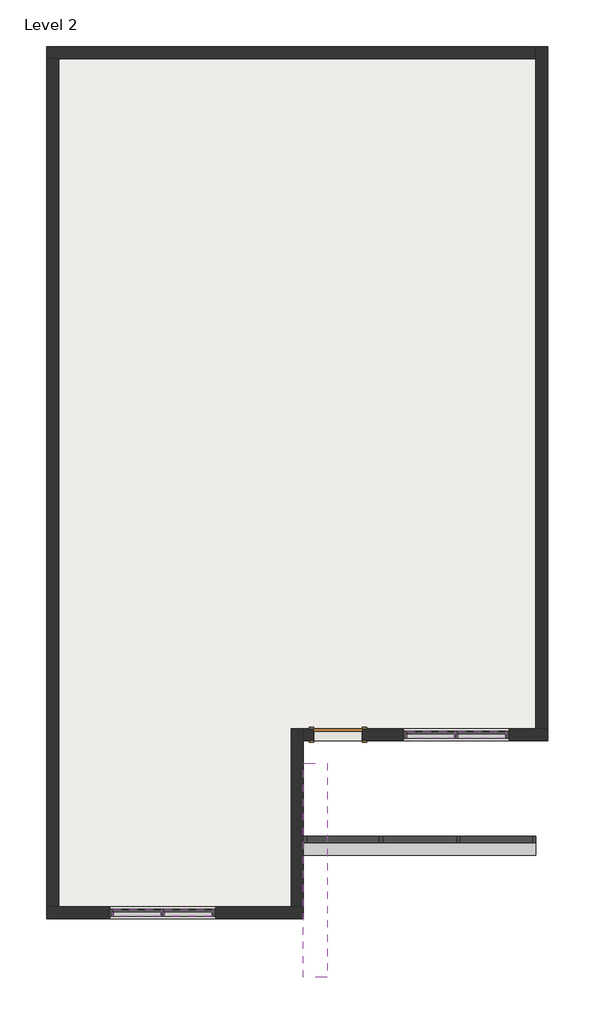
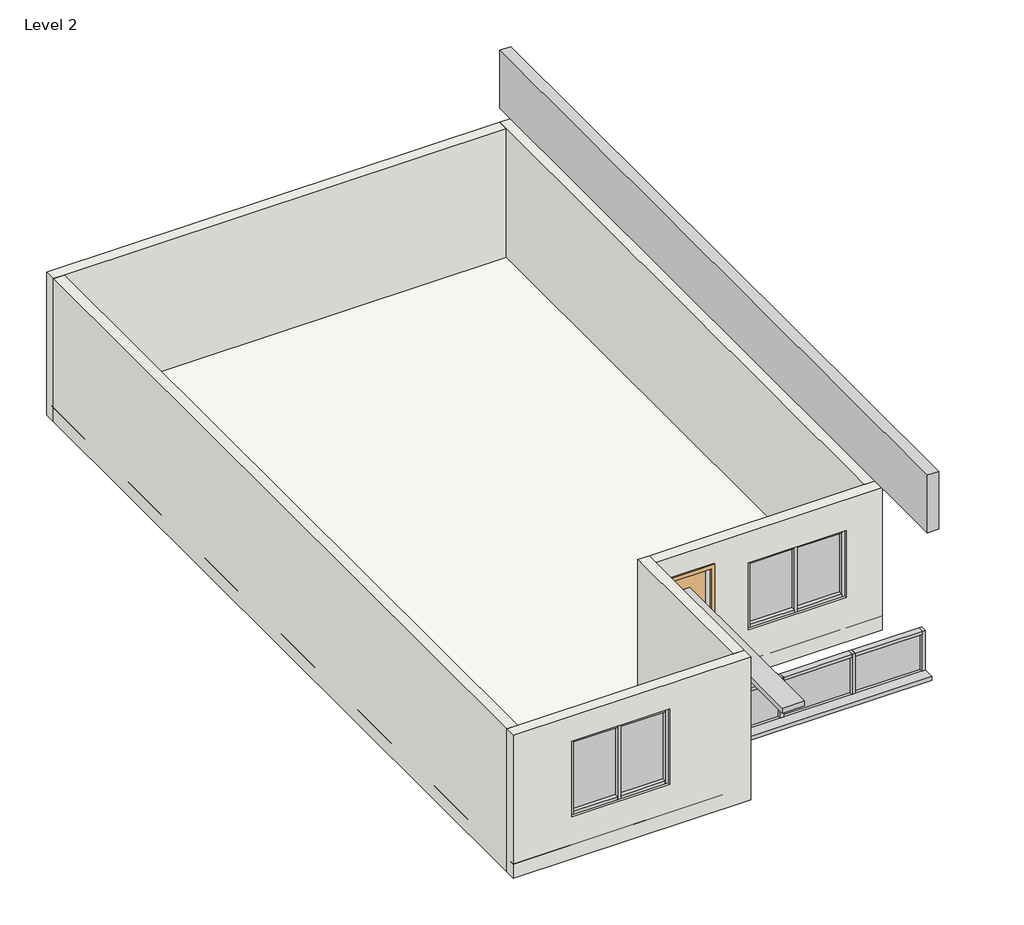
# One storey: 24 members, 7 plates, 6 walls, 2 proxies, 1 door, 1 roof.
"""IFC4 building model written with IfcOpenShell, lengths in millimetres."""

from ifc_helpers import new_model, si_unit, frame, origin, place, context, project, spatial, polyline, outline, extrude, faceted_brep, transform, mapped, element, save
from components import generic_models_2_generic_models_2_9dd516d1, generic_models_3_generic_models_3_6894cc3d, door_0ca8825f, member_f1f71bde, member_1afc5165, member_5bd926c3, member_c72ed4d9, member_c6cbf9be, member_20eb5ac3, member_846957be, member_d3800c19, member_e1cf819f, system_panel_glazed_d3edc084, system_panel_glazed_88eb0887, system_panel_glazed_baedfebd, system_panel_glazed_353e56bd

model = new_model("IFC4")

# Units and contexts
model_context = context("Model", 3, world=origin())
ifc_project = project(units=[si_unit("LENGTHUNIT", "METRE", prefix="MILLI")], contexts=[model_context])

# Site, building, storey
site = spatial("IfcSite", under=ifc_project)
building = spatial("IfcBuilding", under=site)
storey = spatial("IfcBuildingStorey", under=building, Name="Level 2", Elevation=3048.0)

# Proxies
placement = place(None, origin())
generic_models_2_generic_models_2_shape = generic_models_2_generic_models_2_9dd516d1(model_context)
element("IfcBuildingElementProxy", 1, Name="Generic Models 2 : Generic Models 2", ObjectType="Generic Models 2 : Generic Models 2", at=placement, inside=storey, context=model_context, shape_type="MappedRepresentation", body=[
    mapped(generic_models_2_generic_models_2_shape, transform((0.0, 0.0, 0.0), x_axis=(1.0, 0.0, 0.0), y_axis=(0.0, 1.0, 0.0), z_axis=(0.0, 0.0, 1.0))),
])
generic_models_3_generic_models_3_shape = generic_models_3_generic_models_3_6894cc3d(model_context)
element("IfcBuildingElementProxy", 2, Name="Generic Models 3 : Generic Models 3", ObjectType="Generic Models 3 : Generic Models 3", at=placement, inside=storey, context=model_context, shape_type="MappedRepresentation", body=[
    mapped(generic_models_3_generic_models_3_shape, transform((0.0, 0.0, 0.0), x_axis=(1.0, 0.0, 0.0), y_axis=(0.0, 1.0, 0.0), z_axis=(0.0, 0.0, 1.0))),
])

# Door
door_shape = door_0ca8825f(model_context)
element("IfcDoor", 3, ObjectType="Single-Flush : 36\" x 84\"", at=placement, inside=storey, context=model_context, shape_type="MappedRepresentation", body=[
    mapped(door_shape, transform((-14644.7161422, -7377.2867758, 3454.4), x_axis=(1.0, 0.0, 0.0), y_axis=(0.0, 1.0, 0.0), z_axis=(0.0, 0.0, 1.0))),
])

# Members
member_shape = member_f1f71bde(model_context)
element("IfcMember", 4, ObjectType="Rectangular Mullion : 2.5\" x 5\" rectangular", at=placement, inside=storey, context=model_context, shape_type="MappedRepresentation", body=[
    mapped(member_shape, transform((-17889.5661422, -10704.6867758, 3945.1177063), x_axis=(0.0, 0.0, -1.0), y_axis=(0.0, -1.0, 0.0), z_axis=(-1.0, 0.0, 0.0))),
])
element("IfcMember", 5, ObjectType="Rectangular Mullion : 2.5\" x 5\" rectangular", at=placement, inside=storey, context=model_context, shape_type="MappedRepresentation", body=[
    mapped(member_shape, transform((-18848.4161422, -10704.6867758, 3945.1177063), x_axis=(0.0, 0.0, -1.0), y_axis=(0.0, -1.0, 0.0), z_axis=(-1.0, 0.0, 0.0))),
])
element("IfcMember", 6, ObjectType="Rectangular Mullion : 2.5\" x 5\" rectangular", at=placement, inside=storey, context=model_context, shape_type="MappedRepresentation", body=[
    mapped(member_shape, transform((-12403.1661422, -7377.2867758, 3998.6028627), x_axis=(0.0, 0.0, -1.0), y_axis=(0.0, -1.0, 0.0), z_axis=(-1.0, 0.0, 0.0))),
])
element("IfcMember", 7, ObjectType="Rectangular Mullion : 2.5\" x 5\" rectangular", at=placement, inside=storey, context=model_context, shape_type="MappedRepresentation", body=[
    mapped(member_shape, transform((-13362.0161422, -7377.2867758, 3998.6028627), x_axis=(0.0, 0.0, -1.0), y_axis=(0.0, -1.0, 0.0), z_axis=(-1.0, 0.0, 0.0))),
])
element("IfcMember", 8, ObjectType="Rectangular Mullion : 2.5\" x 5\" rectangular", at=placement, inside=storey, context=model_context, shape_type="MappedRepresentation", body=[
    mapped(member_shape, transform((-17953.0661422, -10704.6867758, 5554.6402073), x_axis=(0.0, 0.0, 1.0), y_axis=(0.0, -1.0, 0.0), z_axis=(1.0, 0.0, 0.0))),
])
element("IfcMember", 9, ObjectType="Rectangular Mullion : 2.5\" x 5\" rectangular", at=placement, inside=storey, context=model_context, shape_type="MappedRepresentation", body=[
    mapped(member_shape, transform((-16994.2161422, -10704.6867758, 5554.6402073), x_axis=(0.0, 0.0, 1.0), y_axis=(0.0, -1.0, 0.0), z_axis=(1.0, 0.0, 0.0))),
])
element("IfcMember", 10, ObjectType="Rectangular Mullion : 2.5\" x 5\" rectangular", at=placement, inside=storey, context=model_context, shape_type="MappedRepresentation", body=[
    mapped(member_shape, transform((-12466.6661422, -7377.2867758, 5431.5526731), x_axis=(0.0, 0.0, 1.0), y_axis=(0.0, -1.0, 0.0), z_axis=(1.0, 0.0, 0.0))),
])
element("IfcMember", 11, ObjectType="Rectangular Mullion : 2.5\" x 5\" rectangular", at=placement, inside=storey, context=model_context, shape_type="MappedRepresentation", body=[
    mapped(member_shape, transform((-11507.8161422, -7377.2867758, 5431.5526731), x_axis=(0.0, 0.0, 1.0), y_axis=(0.0, -1.0, 0.0), z_axis=(1.0, 0.0, 0.0))),
])
member_2_shape = member_1afc5165(model_context)
element("IfcMember", 12, ObjectType="Rectangular Mullion : 2.5\" x 5\" rectangular", at=placement, inside=storey, context=model_context, shape_type="MappedRepresentation", body=[
    mapped(member_2_shape, transform((-17921.3161422, -10704.6867758, 3945.1177063), x_axis=(1.0, 0.0, 0.0), y_axis=(0.0, -1.0, 0.0), z_axis=(0.0, 0.0, -1.0))),
])
member_3_shape = member_5bd926c3(model_context)
element("IfcMember", 13, ObjectType="Rectangular Mullion : 2.5\" x 5\" rectangular", at=placement, inside=storey, context=model_context, shape_type="MappedRepresentation", body=[
    mapped(member_3_shape, transform((-18911.9161422, -10704.6867758, 5554.6402073), x_axis=(-1.0, 0.0, 0.0), y_axis=(0.0, -1.0, 0.0), z_axis=(0.0, 0.0, 1.0))),
])
element("IfcMember", 14, ObjectType="Rectangular Mullion : 2.5\" x 5\" rectangular", at=placement, inside=storey, context=model_context, shape_type="MappedRepresentation", body=[
    mapped(member_3_shape, transform((-16930.7161422, -10704.6867758, 3945.1177063), x_axis=(1.0, 0.0, 0.0), y_axis=(0.0, -1.0, 0.0), z_axis=(0.0, 0.0, -1.0))),
])
member_4_shape = member_c72ed4d9(model_context)
element("IfcMember", 15, ObjectType="Rectangular Mullion : 2.5\" x 5\" rectangular", at=placement, inside=storey, context=model_context, shape_type="MappedRepresentation", body=[
    mapped(member_4_shape, transform((-12434.9161422, -7377.2867758, 3998.6028627), x_axis=(1.0, 0.0, 0.0), y_axis=(0.0, -1.0, 0.0), z_axis=(0.0, 0.0, -1.0))),
])
member_5_shape = member_c6cbf9be(model_context)
element("IfcMember", 16, ObjectType="Rectangular Mullion : 2.5\" x 5\" rectangular", at=placement, inside=storey, context=model_context, shape_type="MappedRepresentation", body=[
    mapped(member_5_shape, transform((-13425.5161422, -7377.2867758, 5431.5526731), x_axis=(-1.0, 0.0, 0.0), y_axis=(0.0, -1.0, 0.0), z_axis=(0.0, 0.0, 1.0))),
])
element("IfcMember", 17, ObjectType="Rectangular Mullion : 2.5\" x 5\" rectangular", at=placement, inside=storey, context=model_context, shape_type="MappedRepresentation", body=[
    mapped(member_5_shape, transform((-11444.3161422, -7377.2867758, 3998.6028627), x_axis=(1.0, 0.0, 0.0), y_axis=(0.0, -1.0, 0.0), z_axis=(0.0, 0.0, -1.0))),
])
member_6_shape = member_20eb5ac3(model_context)
element("IfcMember", 18, ObjectType="Rectangular Mullion : 2.5\" x 5\" rectangular", at=placement, inside=storey, context=model_context, shape_type="MappedRepresentation", body=[
    mapped(member_6_shape, transform((-13876.3661422, -9333.0867758, 4278.7054943), x_axis=(0.0, 0.0, 1.0), y_axis=(0.0, -1.0, 0.0), z_axis=(1.0, 0.0, 0.0))),
])
element("IfcMember", 19, ObjectType="Rectangular Mullion : 2.5\" x 5\" rectangular", at=placement, inside=storey, context=model_context, shape_type="MappedRepresentation", body=[
    mapped(member_6_shape, transform((-11012.5161422, -9333.0867758, 4278.7054943), x_axis=(0.0, 0.0, 1.0), y_axis=(0.0, -1.0, 0.0), z_axis=(1.0, 0.0, 0.0))),
])
member_7_shape = member_846957be(model_context)
element("IfcMember", 20, ObjectType="Rectangular Mullion : 2.5\" x 5\" rectangular", at=placement, inside=storey, context=model_context, shape_type="MappedRepresentation", body=[
    mapped(member_7_shape, transform((-13844.6161422, -9333.0867758, 3352.8), x_axis=(1.0, 0.0, 0.0), y_axis=(0.0, -1.0, 0.0), z_axis=(0.0, 0.0, -1.0))),
])
element("IfcMember", 21, ObjectType="Rectangular Mullion : 2.5\" x 5\" rectangular", at=placement, inside=storey, context=model_context, shape_type="MappedRepresentation", body=[
    mapped(member_7_shape, transform((-12396.8161422, -9333.0867758, 3352.8), x_axis=(1.0, 0.0, 0.0), y_axis=(0.0, -1.0, 0.0), z_axis=(0.0, 0.0, -1.0))),
])
element("IfcMember", 22, ObjectType="Rectangular Mullion : 2.5\" x 5\" rectangular", at=placement, inside=storey, context=model_context, shape_type="MappedRepresentation", body=[
    mapped(member_6_shape, transform((-12365.0661422, -9333.0867758, 3352.8), x_axis=(0.0, 0.0, -1.0), y_axis=(0.0, -1.0, 0.0), z_axis=(-1.0, 0.0, 0.0))),
])
element("IfcMember", 23, ObjectType="Rectangular Mullion : 2.5\" x 5\" rectangular", at=placement, inside=storey, context=model_context, shape_type="MappedRepresentation", body=[
    mapped(member_6_shape, transform((-15228.9161422, -9333.0867758, 3352.8), x_axis=(0.0, 0.0, -1.0), y_axis=(0.0, -1.0, 0.0), z_axis=(-1.0, 0.0, 0.0))),
])
member_8_shape = member_d3800c19(model_context)
element("IfcMember", 24, ObjectType="Rectangular Mullion : 2.5\" x 5\" rectangular", at=placement, inside=storey, context=model_context, shape_type="MappedRepresentation", body=[
    mapped(member_8_shape, transform((-15292.4161422, -9333.0867758, 4278.7054943), x_axis=(-1.0, 0.0, 0.0), y_axis=(0.0, -1.0, 0.0), z_axis=(0.0, 0.0, 1.0))),
])
member_9_shape = member_e1cf819f(model_context)
element("IfcMember", 25, ObjectType="Rectangular Mullion : 2.5\" x 5\" rectangular", at=placement, inside=storey, context=model_context, shape_type="MappedRepresentation", body=[
    mapped(member_9_shape, transform((-12428.5661422, -9333.0867758, 4278.7054943), x_axis=(0.0, 0.0, 1.0), y_axis=(0.0, -1.0, 0.0), z_axis=(1.0, 0.0, 0.0))),
])
element("IfcMember", 26, ObjectType="Rectangular Mullion : 2.5\" x 5\" rectangular", at=placement, inside=storey, context=model_context, shape_type="MappedRepresentation", body=[
    mapped(member_9_shape, transform((-13812.8661422, -9333.0867758, 3352.8), x_axis=(0.0, 0.0, -1.0), y_axis=(0.0, -1.0, 0.0), z_axis=(-1.0, 0.0, 0.0))),
])
element("IfcMember", 27, ObjectType="Rectangular Mullion : 2.5\" x 5\" rectangular", at=placement, inside=storey, context=model_context, shape_type="MappedRepresentation", body=[
    mapped(member_8_shape, transform((-10949.0161422, -9333.0867758, 3352.8), x_axis=(1.0, 0.0, 0.0), y_axis=(0.0, -1.0, 0.0), z_axis=(0.0, 0.0, -1.0))),
])

# Plates
system_panel_glazed_shape = system_panel_glazed_d3edc084(model_context)
element("IfcPlate", 28, ObjectType="System Panel : Glazed", at=placement, inside=storey, context=model_context, shape_type="MappedRepresentation", body=[
    mapped(system_panel_glazed_shape, transform((-18400.7411422, -10704.6867758, 4008.6177063), x_axis=(1.0, 0.0, 0.0), y_axis=(0.0, 1.0, 0.0), z_axis=(0.0, 0.0, 1.0))),
])
element("IfcPlate", 29, ObjectType="System Panel : Glazed", at=placement, inside=storey, context=model_context, shape_type="MappedRepresentation", body=[
    mapped(system_panel_glazed_shape, transform((-17441.8911422, -10704.6867758, 4008.6177063), x_axis=(1.0, 0.0, 0.0), y_axis=(0.0, 1.0, 0.0), z_axis=(0.0, 0.0, 1.0))),
])
system_panel_glazed_2_shape = system_panel_glazed_88eb0887(model_context)
element("IfcPlate", 30, ObjectType="System Panel : Glazed", at=placement, inside=storey, context=model_context, shape_type="MappedRepresentation", body=[
    mapped(system_panel_glazed_2_shape, transform((-12914.3411422, -7377.2867758, 4062.1028627), x_axis=(1.0, 0.0, 0.0), y_axis=(0.0, 1.0, 0.0), z_axis=(0.0, 0.0, 1.0))),
])
element("IfcPlate", 31, ObjectType="System Panel : Glazed", at=placement, inside=storey, context=model_context, shape_type="MappedRepresentation", body=[
    mapped(system_panel_glazed_2_shape, transform((-11955.4911422, -7377.2867758, 4062.1028627), x_axis=(1.0, 0.0, 0.0), y_axis=(0.0, 1.0, 0.0), z_axis=(0.0, 0.0, 1.0))),
])
system_panel_glazed_3_shape = system_panel_glazed_baedfebd(model_context)
element("IfcPlate", 32, ObjectType="System Panel : Glazed", at=placement, inside=storey, context=model_context, shape_type="MappedRepresentation", body=[
    mapped(system_panel_glazed_3_shape, transform((-14552.6411422, -9333.0867758, 3416.3), x_axis=(1.0, 0.0, 0.0), y_axis=(0.0, 1.0, 0.0), z_axis=(0.0, 0.0, 1.0))),
])
element("IfcPlate", 33, ObjectType="System Panel : Glazed", at=placement, inside=storey, context=model_context, shape_type="MappedRepresentation", body=[
    mapped(system_panel_glazed_3_shape, transform((-11688.7911422, -9333.0867758, 3416.3), x_axis=(1.0, 0.0, 0.0), y_axis=(0.0, 1.0, 0.0), z_axis=(0.0, 0.0, 1.0))),
])
system_panel_glazed_4_shape = system_panel_glazed_353e56bd(model_context)
element("IfcPlate", 34, ObjectType="System Panel : Glazed", at=placement, inside=storey, context=model_context, shape_type="MappedRepresentation", body=[
    mapped(system_panel_glazed_4_shape, transform((-13120.7161422, -9333.0867758, 3416.3), x_axis=(1.0, 0.0, 0.0), y_axis=(0.0, 1.0, 0.0), z_axis=(0.0, 0.0, 1.0))),
])

# Roof
element("IfcRoof", 35, ObjectType="Generic - 12\"", at=placement, inside=storey, context=model_context, shape_type="SweptSolid", body=[
    extrude(outline(polyline([(-20093.0161422, 5487.8132242), (-10720.4161422, 5487.8132242), (-10720.4161422, -7491.5867758), (-15292.4161422, -7491.5867758), (-15292.4161422, -10539.5867758), (-15292.4161422, -10818.9867758), (-20093.0161422, -10818.9867758), (-20093.0161422, -10590.3867758), (-20093.0161422, 5487.8132242)])), frame((0.0, 0.0, 3048.0), z_axis=(0.0, 0.0, 1.0), x_axis=(1.0, 0.0, 0.0)), (0.0, 0.0, 1.0), 304.8),
])

# Walls
element("IfcWall", 36, ObjectType="9\"", at=placement, inside=storey, context=model_context, shape_type="Brep", body=[
    faceted_brep([(-20093.0161422, -10818.9867758, 3048.0), (-15292.4161422, -10818.9867758, 3048.0), (-15292.4161422, -10818.9867758, 6096.0), (-20093.0161422, -10818.9867758, 6096.0), (-18911.9161422, -10818.9867758, 3945.1177063), (-18911.9161422, -10818.9867758, 5554.6402073), (-16930.7161422, -10818.9867758, 5554.6402073), (-16930.7161422, -10818.9867758, 3945.1177063), (-15292.4161422, -10590.3867758, 3048.0), (-15521.0161422, -10590.3867758, 3048.0), (-19864.4161422, -10590.3867758, 3048.0), (-20093.0161422, -10590.3867758, 3048.0), (-20093.0161422, -10590.3867758, 6096.0), (-19864.4161422, -10590.3867758, 6096.0), (-15521.0161422, -10590.3867758, 6096.0), (-15292.4161422, -10590.3867758, 6096.0), (-18911.9161422, -10590.3867758, 5554.6402073), (-18911.9161422, -10590.3867758, 3945.1177063), (-16930.7161422, -10590.3867758, 3945.1177063), (-16930.7161422, -10590.3867758, 5554.6402073)], [[[0, 1, 2, 3], [4, 5, 6, 7]], [[8, 9, 10, 11, 12, 13, 14, 15], [16, 17, 18, 19]], [[1, 0, 11, 10, 9, 8]], [[3, 2, 15, 14, 13, 12]], [[2, 1, 8, 15]], [[0, 3, 12, 11]], [[4, 17, 16, 5]], [[5, 16, 19, 6]], [[6, 19, 18, 7]], [[17, 4, 7, 18]]]),
])
element("IfcWall", 37, ObjectType="9\"", at=placement, inside=storey, context=model_context, shape_type="Brep", body=[
    faceted_brep([(-15292.4161422, -10590.3867758, 3048.0), (-15292.4161422, -7491.5867758, 3048.0), (-15292.4161422, -7262.9867758, 3048.0), (-15292.4161422, -7262.9867758, 6096.0), (-15292.4161422, -7491.5867758, 6096.0), (-15292.4161422, -10590.3867758, 6096.0), (-15521.0161422, -10590.3867758, 3048.0), (-15521.0161422, -10590.3867758, 6096.0), (-15521.0161422, -7262.9867758, 6096.0), (-15521.0161422, -7262.9867758, 3048.0)], [[[0, 1, 2, 3, 4, 5]], [[6, 7, 8, 9]], [[2, 1, 0, 6, 9]], [[5, 4, 3, 8, 7]], [[0, 5, 7, 6]], [[3, 2, 9, 8]]]),
])
element("IfcWall", 38, ObjectType="9\"", at=placement, inside=storey, context=model_context, shape_type="Brep", body=[
    faceted_brep([(-15292.4161422, -7491.5867758, 3048.0), (-10720.4161422, -7491.5867758, 3048.0), (-10720.4161422, -7491.5867758, 6096.0), (-15292.4161422, -7491.5867758, 6096.0), (-15101.9161422, -7491.5867758, 3454.4), (-15101.9161422, -7491.5867758, 5588.0), (-14187.5161422, -7491.5867758, 5588.0), (-14187.5161422, -7491.5867758, 3454.4), (-13425.5161422, -7491.5867758, 3998.6028627), (-13425.5161422, -7491.5867758, 5431.5526731), (-11444.3161422, -7491.5867758, 5431.5526731), (-11444.3161422, -7491.5867758, 3998.6028627), (-10720.4161422, -7262.9867758, 3048.0), (-10949.0161422, -7262.9867758, 3048.0), (-15292.4161422, -7262.9867758, 3048.0), (-15292.4161422, -7262.9867758, 6096.0), (-10949.0161422, -7262.9867758, 6096.0), (-10720.4161422, -7262.9867758, 6096.0), (-15101.9161422, -7262.9867758, 3454.4), (-14187.5161422, -7262.9867758, 3454.4), (-14187.5161422, -7262.9867758, 5588.0), (-15101.9161422, -7262.9867758, 5588.0), (-13425.5161422, -7262.9867758, 5431.5526731), (-13425.5161422, -7262.9867758, 3998.6028627), (-11444.3161422, -7262.9867758, 3998.6028627), (-11444.3161422, -7262.9867758, 5431.5526731)], [[[0, 1, 2, 3], [4, 5, 6, 7], [8, 9, 10, 11]], [[12, 13, 14, 15, 16, 17], [18, 19, 20, 21], [22, 23, 24, 25]], [[1, 0, 14, 13, 12]], [[3, 2, 17, 16, 15]], [[0, 3, 15, 14]], [[2, 1, 12, 17]], [[19, 18, 4, 7]], [[20, 19, 7, 6]], [[21, 20, 6, 5]], [[18, 21, 5, 4]], [[8, 23, 22, 9]], [[9, 22, 25, 10]], [[10, 25, 24, 11]], [[23, 8, 11, 24]]]),
])
element("IfcWall", 39, ObjectType="9\"", at=placement, inside=storey, context=model_context, shape_type="Brep", body=[
    faceted_brep([(-10720.4161422, -7262.9867758, 3048.0), (-10720.4161422, 5487.8132242, 3048.0), (-10720.4161422, 5487.8132242, 6096.0), (-10720.4161422, -7262.9867758, 6096.0), (-10949.0161422, -7262.9867758, 3048.0), (-10949.0161422, -7262.9867758, 6096.0), (-10949.0161422, 5259.2132242, 6096.0), (-10949.0161422, 5487.8132242, 6096.0), (-10949.0161422, 5487.8132242, 3048.0), (-10949.0161422, 5259.2132242, 3048.0)], [[[0, 1, 2, 3]], [[4, 5, 6, 7, 8, 9]], [[1, 0, 4, 9, 8]], [[3, 2, 7, 6, 5]], [[0, 3, 5, 4]], [[2, 1, 8, 7]]]),
])
element("IfcWall", 40, ObjectType="9\"", at=placement, inside=storey, context=model_context, shape_type="Brep", body=[
    faceted_brep([(-10949.0161422, 5487.8132242, 3048.0), (-20093.0161422, 5487.8132242, 3048.0), (-20093.0161422, 5487.8132242, 6096.0), (-10949.0161422, 5487.8132242, 6096.0), (-10949.0161422, 5259.2132242, 3048.0), (-10949.0161422, 5259.2132242, 6096.0), (-19864.4161422, 5259.2132242, 6096.0), (-20093.0161422, 5259.2132242, 6096.0), (-20093.0161422, 5259.2132242, 3048.0), (-19864.4161422, 5259.2132242, 3048.0)], [[[0, 1, 2, 3]], [[4, 5, 6, 7, 8, 9]], [[1, 0, 4, 9, 8]], [[3, 2, 7, 6, 5]], [[0, 3, 5, 4]], [[2, 1, 8, 7]]]),
])
element("IfcWall", 41, ObjectType="9\"", at=placement, inside=storey, context=model_context, shape_type="SweptSolid", body=[
    extrude(outline(polyline([(-20093.0161422, -10590.3867758), (-20093.0161422, 5259.2132242), (-19864.4161422, 5259.2132242), (-19864.4161422, -10590.3867758), (-20093.0161422, -10590.3867758)])), frame((0.0, 0.0, 3048.0), z_axis=(0.0, 0.0, 1.0), x_axis=(1.0, 0.0, 0.0)), (0.0, 0.0, 1.0), 3048.0),
])

save(model, "model.ifc")

# Revit data of these elements
# Type "Single-Flush : 36\" x 84\""
#   Type Mark = "1"
#   Construction Type Id = "MDOOR"
#   Assembly Code = "C1020"
#   Analytic Construction = "Metal"
#   Thickness = 0' - 2"
#   Heat Transfer Coefficient (U) = 0.651978 BTU/(h·ft²·°F)
#   Height = 7' - 0"
#   Trim Projection Ext = 0' - 1"
#   Trim Projection Int = 0' - 1"
#   Trim Width = 0' - 3"
#   Width = 3' - 0"
#   Define Thermal Properties by = 1
#   Define Thermal Properties by = 1
#   Door Material = Door - Panel
#   Frame Material = Door - Frame
#   Visual Light Transmittance = 0
#   Solar Heat Gain Coefficient = 0
#   Function = (empty or 0)
#   Wall Closure = (empty or 0)
# Type "Rectangular Mullion : 2.5\" x 5\" rectangular"
#   built-in parameter 1007304 = 0.416667 (stored number, unit not read)
#   built-in parameter 1007301 = 0.104167 (stored number, unit not read)
#   built-in parameter 1007300 = 0.104167 (stored number, unit not read)
# Type "System Panel : Glazed"
#   Construction Type Id = "GSP4R"
#   Analytic Construction = "1/8 in Pilkington single glazing"
#   Visual Light Transmittance = 0.9
#   Solar Heat Gain Coefficient = 0.86
#   Heat Transfer Coefficient (U) = 1.18115 BTU/(h·ft²·°F)
#   Define Thermal Properties by = 1
# Type "Generic - 12\""
#   Assembly Code = "B1020"
#   Layers, outside or top first: 1' - 0" no material (function 1)
# Type "9\""
#   Assembly Code = "B2010"
#   Layers, outside or top first: 0' - 9" no material (function 1)
# Element 1 (IfcBuildingElementProxy, "Generic Models 2 : Generic Models 2")
#   Phase Created = New Construction
# Element 2 (IfcBuildingElementProxy, "Generic Models 3 : Generic Models 3")
#   Phase Created = New Construction
# Element 3 (IfcDoor, "Single-Flush : 36\" x 84\"")
#   Phase Created = New Construction
#   Materials on its faces: "Door - Frame", "Door - Panel"
# Elements 4, 5, 6, 7, 8, 9, 10, 11, 12, 13, 14, 15, 16, 17, 18, 19, 20, 21, 22, 23, 24, 25, 26, 27 (IfcMember, "Rectangular Mullion : 2.5\" x 5\" rectangular")
#   Phase Created = New Construction
#   Materials on its faces: "Aluminum"
# Elements 28, 29, 30, 31, 32, 33, 34 (IfcPlate, "System Panel : Glazed")
#   Phase Created = New Construction
#   Materials on its faces: "Glass"
# Element 35 (IfcRoof, "Generic - 12\"")
#   built-in parameter 1001705 = 11 (stored number, unit not read)
#   built-in parameter 1001710 = 33615
#   Phase Created = New Construction
#   Materials on its faces: "Default Roof"
# Elements 36, 37, 38, 39, 40, 41 (IfcWall, "9\"")
#   Top Offset = 0' - 0"
#   Base Offset = 0' - 0"
#   Unconnected Height = 10' - 0"
#   wall height = 10' - 0"
#   Phase Created = New Construction
#   Base Constraint = Level 2
#   Materials on its faces: "Default Wall"
# Materials
#   "Door - Panel": class "Wood", colour RGB 210 159 95, transparency 0, Cost = 0
#   "Door - Frame": colour RGB 118 70 51, transparency 0, Cost = 0
#   "Aluminum": class "Metal", colour RGB 247 247 247, transparency 0, Description = "Aluminum 6061", Cost = 0
#   "Glass": class "Glass", colour RGB 0 128 192, transparency 0.75, Description = "Soda Lime Glass", Cost = 0
#   "Default Roof": colour RGB 88 101 114, transparency 0, Cost = 0
#   "Default Wall": colour RGB 128 128 128, transparency 0, Cost = 0
